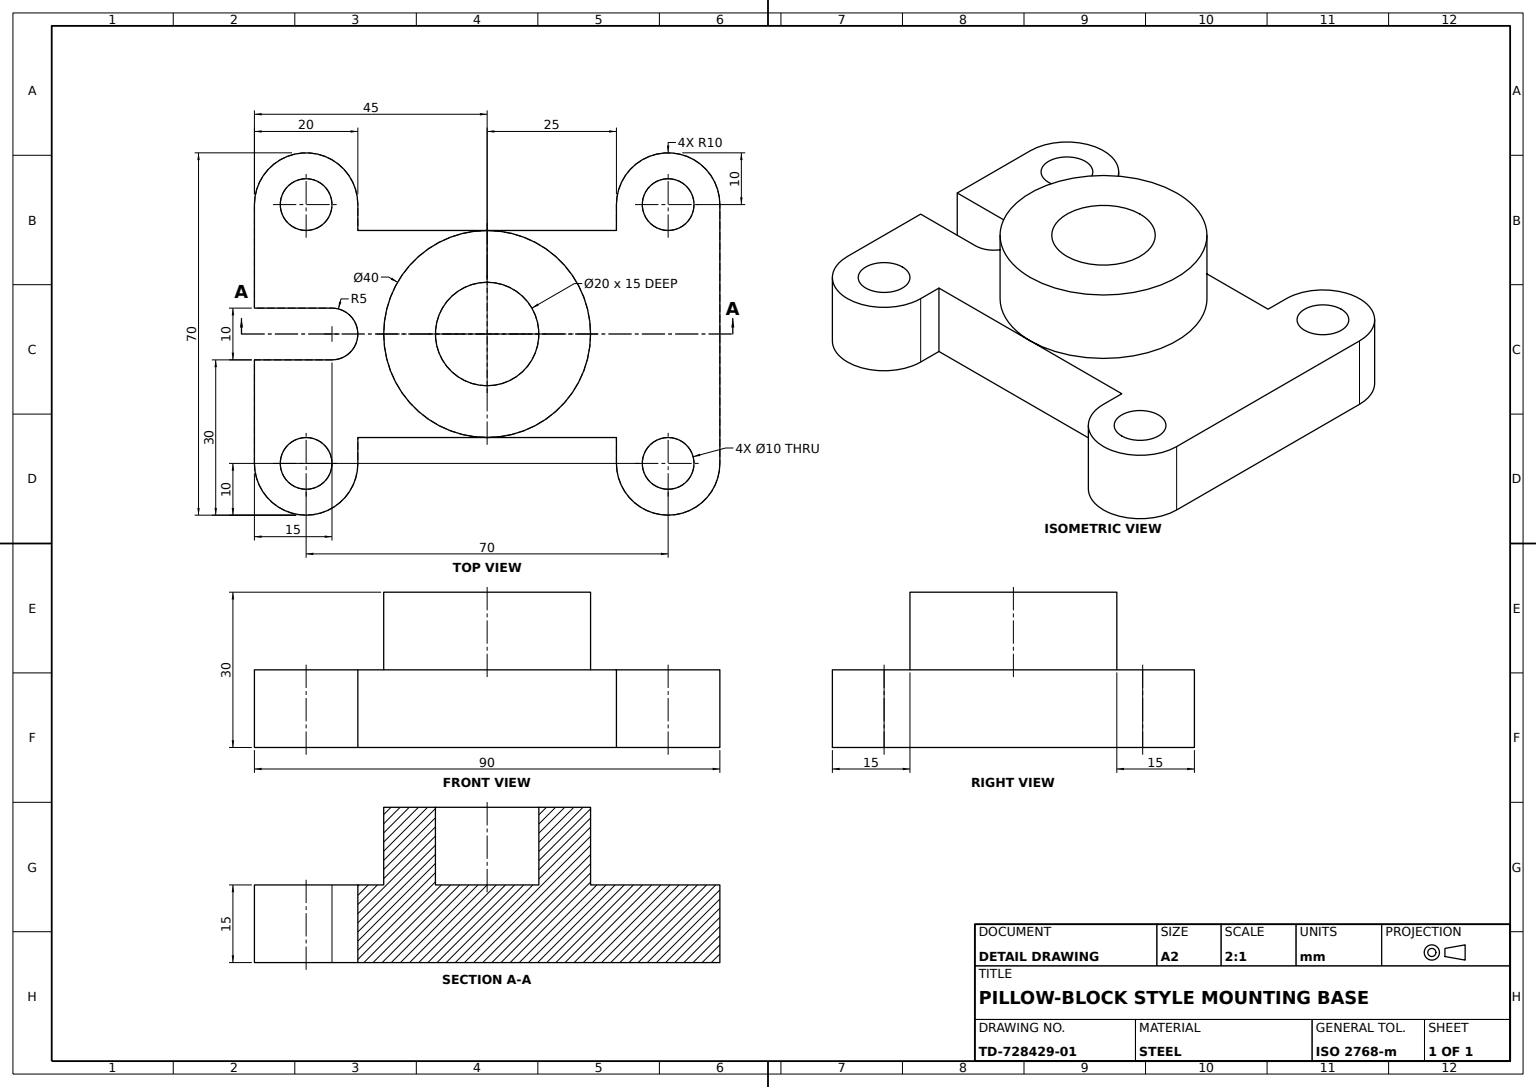
SolidWorks part; units mm, degrees
material "Plain Carbon Steel"
ref_plane "Front Plane" through (0, 0, 0) normal (0, 0, 1) x (1, 0, 0)
ref_plane "Top Plane" through (0, 0, 0) normal (0, 1, 0) x (1, 0, 0)
ref_plane "Right Plane" through (0, 0, 0) normal (1, 0, 0) x (0, 0, -1)
sketch "Base Plate Sketch" plane through (0, 0, 0) normal (0, 1, 0) x (1, 0, 0)
  line L0 (-25, 20) -> (25, 20)
  line L1 (35, 20) -> (35, 25)
  line L2 (0, 0) -> (0, 41.9907) construction
  line L3 (45, 25) -> (45, -25)
  line L10 (-45, 25) -> (-45, 5)
  line L11 (-56.7734, 0) -> (-30, 0) construction
  line L12 (-45, -5) -> (-30, -5)
  line L13 (-45, 5) -> (-30, 5)
  line L14 (-45, -5) -> (-45, -25)
  line L17 (25, 25) -> (25, 20)
  line L18 (25, -25) -> (25, -20)
  line L20 (-25, 25) -> (-25, 20)
  line L21 (-25, -25) -> (-25, -20)
  line L22 (-25, -20) -> (25, -20)
  circle A0 centre (35, 25) radius 5
  circle A1 centre (-35, 25) radius 5
  arc A3 (-45, 25) -> (-25, 25) centre (-35, 25) cw
  circle A4 centre (-35, -25) radius 5
  arc A5 (-45, -25) -> (-25, -25) centre (-35, -25) ccw
  circle A6 centre (35, -25) radius 5
  arc A7 (45, -25) -> (25, -25) centre (35, -25) cw
  arc A8 (-30, -5) -> (-30, 5) centre (-30, 0) ccw
  arc A10 (45, 25) -> (25, 25) centre (35, 25) ccw
  point P20 (0, 20)
  point P25 (0, 20)
  dimension "D1" = 5
  dimension "D2" = 5
  dimension "D8" = 10
  dimension "D9" = 10
  dimension "D11" = 10
  dimension "D13" = 10
  dimension "D3" = 70
  dimension "D4" = 15
  dimension "D5" = 25
extrude "Base Plate" add sketch "Base Plate Sketch" against normal blind 15 contours L3 A10 L17 L0 L20 A3 L10 L13 A8 L12 L14 A5 L21 L22 L18 A7 A6 A4 A0 A1
sketch "Pivot Boss Sketch" plane through (0, 0, 0) normal (0, 1, 0) x (1, 0, 0)
  circle A0 centre (0, 0) radius 20
  circle A1 centre (0, 0) radius 10
  dimension "D1" = 40
  dimension "D2" = 20
extrude "Pivot Boss Ø40 Bore Ø20" add sketch "Pivot Boss Sketch" along normal blind 15
